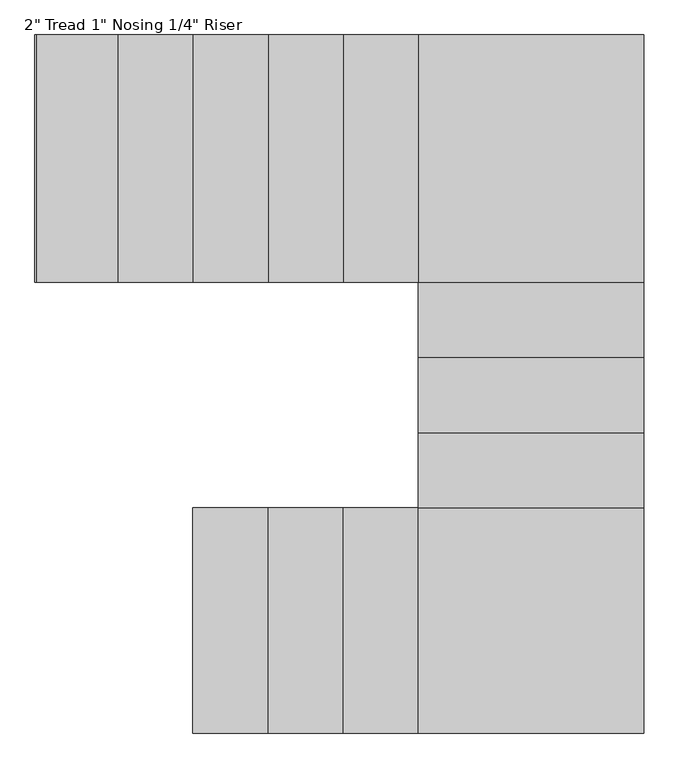
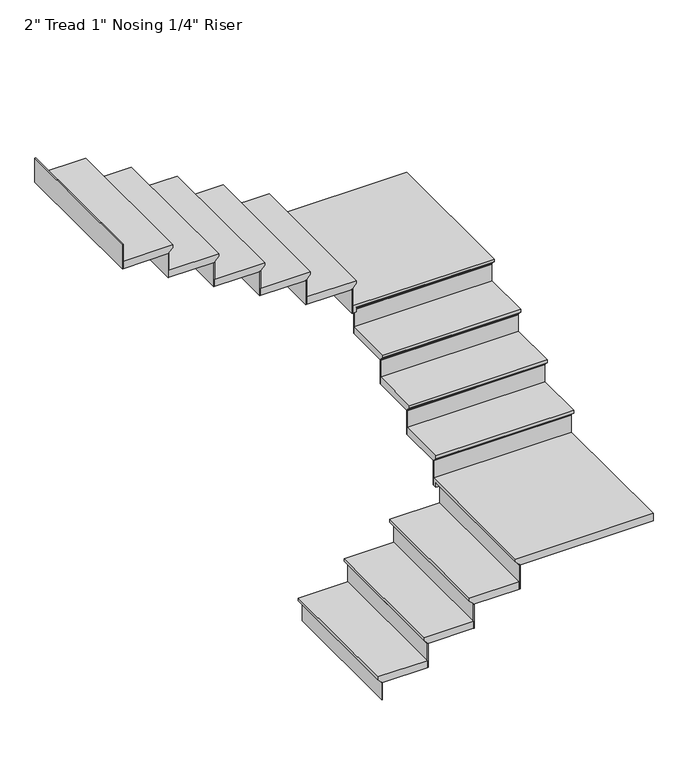
"""IFC4 building model written with IfcOpenShell, lengths in millimetres: stair flight geometry."""

from ifc_helpers import new_model, si_unit, origin, place, context, project, spatial, faceted_brep, source, transform, mapped, element, save


def stair_flight_4ba9adf8(model_context):
    return source(origin(), model_context, "Body", "Brep", [
        faceted_brep([(938.5174794, -182.0870507, 9751.4833333), (938.5174794, -182.0870507, 9770.5333333), (938.5174794, 732.3129493, 9770.5333333), (938.5174794, 732.3129493, 9751.4833333), (963.9174794, -182.0870507, 9726.0833333), (963.9174794, 732.3129493, 9726.0833333), (1268.7174794, -182.0870507, 9770.5333333), (1268.7174794, 732.3129493, 9770.5333333), (963.9174794, 732.3129493, 9719.7333333), (1268.7174794, 732.3129493, 9719.7333333), (1268.7174794, -182.0870507, 9719.7333333), (963.9174794, -182.0870507, 9719.7333333)], [[[0, 1, 2, 3]], [[4, 0, 3, 5]], [[2, 1, 6, 7]], [[8, 9, 10, 11]], [[2, 7, 9, 8, 5, 3]], [[8, 11, 4, 5]], [[6, 1, 0, 4, 11, 10]], [[7, 6, 10, 9]]]),
        faceted_brep([(963.9174794, -182.0870507, 9719.7333333), (963.9174794, -182.0870507, 9601.2), (970.2674794, -182.0870507, 9601.2), (970.2674794, -182.0870507, 9719.7333333), (963.9174794, 732.3129493, 9719.7333333), (970.2674794, 732.3129493, 9719.7333333), (970.2674794, 732.3129493, 9601.2), (963.9174794, 732.3129493, 9601.2)], [[[0, 1, 2, 3]], [[4, 5, 6, 7]], [[1, 0, 4, 7]], [[2, 1, 7, 6]], [[3, 2, 6, 5]], [[0, 3, 5, 4]]]),
        faceted_brep([(1268.7174794, -182.0870507, 9889.0666667), (1268.7174794, -182.0870507, 9719.7333333), (1275.0674794, -182.0870507, 9719.7333333), (1275.0674794, -182.0870507, 9889.0666667), (1268.7174794, 732.3129493, 9889.0666667), (1275.0674794, 732.3129493, 9889.0666667), (1275.0674794, 732.3129493, 9719.7333333), (1268.7174794, 732.3129493, 9719.7333333)], [[[0, 1, 2, 3]], [[4, 5, 6, 7]], [[1, 0, 4, 7]], [[2, 1, 7, 6]], [[3, 2, 6, 5]], [[0, 3, 5, 4]]]),
        faceted_brep([(1243.3174794, 732.3129493, 9939.8666667), (1243.3174794, -182.0870507, 9939.8666667), (1573.5174794, -182.0870507, 9939.8666667), (1573.5174794, 732.3129493, 9939.8666667), (1268.7174794, 732.3129493, 9889.0666667), (1573.5174794, 732.3129493, 9889.0666667), (1573.5174794, -182.0870507, 9889.0666667), (1268.7174794, -182.0870507, 9889.0666667), (1268.7174794, 732.3129493, 9895.4166667), (1243.3174794, 732.3129493, 9920.8166667), (1268.7174794, -182.0870507, 9895.4166667), (1243.3174794, -182.0870507, 9920.8166667)], [[[0, 1, 2, 3]], [[4, 5, 6, 7]], [[0, 3, 5, 4, 8, 9]], [[4, 7, 10, 8]], [[2, 1, 11, 10, 7, 6]], [[3, 2, 6, 5]], [[11, 1, 0, 9]], [[10, 11, 9, 8]]]),
        faceted_brep([(1573.5174794, -182.0870507, 10058.4), (1573.5174794, -182.0870507, 9889.0666667), (1579.8674794, -182.0870507, 9889.0666667), (1579.8674794, -182.0870507, 10058.4), (1573.5174794, 732.3129493, 10058.4), (1579.8674794, 732.3129493, 10058.4), (1579.8674794, 732.3129493, 9889.0666667), (1573.5174794, 732.3129493, 9889.0666667)], [[[0, 1, 2, 3]], [[4, 5, 6, 7]], [[1, 0, 4, 7]], [[2, 1, 7, 6]], [[3, 2, 6, 5]], [[0, 3, 5, 4]]]),
        faceted_brep([(1548.1174794, 732.3129493, 10109.2), (1548.1174794, -182.0870507, 10109.2), (1878.3174794, -182.0870507, 10109.2), (1878.3174794, 732.3129493, 10109.2), (1573.5174794, 732.3129493, 10058.4), (1878.3174794, 732.3129493, 10058.4), (1878.3174794, -182.0870507, 10058.4), (1573.5174794, -182.0870507, 10058.4), (1573.5174794, 732.3129493, 10064.75), (1548.1174794, 732.3129493, 10090.15), (1573.5174794, -182.0870507, 10064.75), (1548.1174794, -182.0870507, 10090.15)], [[[0, 1, 2, 3]], [[4, 5, 6, 7]], [[0, 3, 5, 4, 8, 9]], [[4, 7, 10, 8]], [[2, 1, 11, 10, 7, 6]], [[3, 2, 6, 5]], [[11, 1, 0, 9]], [[10, 11, 9, 8]]]),
        faceted_brep([(1878.3174794, -182.0870507, 10227.7333333), (1878.3174794, -182.0870507, 10058.4), (1884.6674794, -182.0870507, 10058.4), (1884.6674794, -182.0870507, 10227.7333333), (1878.3174794, 732.3129493, 10227.7333333), (1884.6674794, 732.3129493, 10227.7333333), (1884.6674794, 732.3129493, 10058.4), (1878.3174794, 732.3129493, 10058.4)], [[[0, 1, 2, 3]], [[4, 5, 6, 7]], [[1, 0, 4, 7]], [[2, 1, 7, 6]], [[3, 2, 6, 5]], [[0, 3, 5, 4]]]),
        faceted_brep([(2767.3174794, -182.0870507, 10278.5333333), (2767.3174794, 757.7129493, 10278.5333333), (1852.9174794, 757.7129493, 10278.5333333), (1852.9174794, -182.0870507, 10278.5333333), (1852.9174794, 732.3129493, 10227.7333333), (1852.9174794, 757.7129493, 10227.7333333), (2767.3174794, 757.7129493, 10227.7333333), (2767.3174794, -182.0870507, 10227.7333333), (1878.3174794, -182.0870507, 10227.7333333), (1878.3174794, 732.3129493, 10227.7333333), (1852.9174794, 732.3129493, 10259.4833333), (1852.9174794, -182.0870507, 10259.4833333), (1878.3174794, 732.3129493, 10234.0833333), (1878.3174794, -182.0870507, 10234.0833333)], [[[0, 1, 2, 3]], [[4, 5, 6, 7, 8, 9]], [[3, 2, 5, 4, 10, 11]], [[4, 9, 12, 10]], [[9, 8, 13, 12]], [[0, 3, 11, 13, 8, 7]], [[1, 0, 7, 6]], [[2, 1, 6, 5]], [[13, 11, 10, 12]]]),
        faceted_brep([(2767.3174794, 757.7129493, 10397.0666667), (2767.3174794, 757.7129493, 10227.7333333), (2767.3174794, 764.0629493, 10227.7333333), (2767.3174794, 764.0629493, 10397.0666667), (1852.9174794, 757.7129493, 10397.0666667), (1852.9174794, 764.0629493, 10397.0666667), (1852.9174794, 764.0629493, 10227.7333333), (1852.9174794, 757.7129493, 10227.7333333)], [[[0, 1, 2, 3]], [[4, 5, 6, 7]], [[1, 0, 4, 7]], [[2, 1, 7, 6]], [[3, 2, 6, 5]], [[0, 3, 5, 4]]]),
        faceted_brep([(1852.9174794, 732.3129493, 10447.8666667), (2767.3174794, 732.3129493, 10447.8666667), (2767.3174794, 1062.5129493, 10447.8666667), (1852.9174794, 1062.5129493, 10447.8666667), (1852.9174794, 757.7129493, 10397.0666667), (1852.9174794, 1062.5129493, 10397.0666667), (2767.3174794, 1062.5129493, 10397.0666667), (2767.3174794, 757.7129493, 10397.0666667), (1852.9174794, 757.7129493, 10403.4166667), (1852.9174794, 732.3129493, 10428.8166667), (2767.3174794, 757.7129493, 10403.4166667), (2767.3174794, 732.3129493, 10428.8166667)], [[[0, 1, 2, 3]], [[4, 5, 6, 7]], [[0, 3, 5, 4, 8, 9]], [[4, 7, 10, 8]], [[2, 1, 11, 10, 7, 6]], [[3, 2, 6, 5]], [[11, 1, 0, 9]], [[10, 11, 9, 8]]]),
        faceted_brep([(2767.3174794, 1062.5129493, 10566.4), (2767.3174794, 1062.5129493, 10397.0666667), (2767.3174794, 1068.8629493, 10397.0666667), (2767.3174794, 1068.8629493, 10566.4), (1852.9174794, 1062.5129493, 10566.4), (1852.9174794, 1068.8629493, 10566.4), (1852.9174794, 1068.8629493, 10397.0666667), (1852.9174794, 1062.5129493, 10397.0666667)], [[[0, 1, 2, 3]], [[4, 5, 6, 7]], [[1, 0, 4, 7]], [[2, 1, 7, 6]], [[3, 2, 6, 5]], [[0, 3, 5, 4]]]),
        faceted_brep([(1852.9174794, 1037.1129493, 10617.2), (2767.3174794, 1037.1129493, 10617.2), (2767.3174794, 1367.3129493, 10617.2), (1852.9174794, 1367.3129493, 10617.2), (1852.9174794, 1062.5129493, 10566.4), (1852.9174794, 1367.3129493, 10566.4), (2767.3174794, 1367.3129493, 10566.4), (2767.3174794, 1062.5129493, 10566.4), (1852.9174794, 1062.5129493, 10572.75), (1852.9174794, 1037.1129493, 10598.15), (2767.3174794, 1062.5129493, 10572.75), (2767.3174794, 1037.1129493, 10598.15)], [[[0, 1, 2, 3]], [[4, 5, 6, 7]], [[0, 3, 5, 4, 8, 9]], [[4, 7, 10, 8]], [[2, 1, 11, 10, 7, 6]], [[3, 2, 6, 5]], [[11, 1, 0, 9]], [[10, 11, 9, 8]]]),
        faceted_brep([(2767.3174794, 1367.3129493, 10735.7333333), (2767.3174794, 1367.3129493, 10566.4), (2767.3174794, 1373.6629493, 10566.4), (2767.3174794, 1373.6629493, 10735.7333333), (1852.9174794, 1367.3129493, 10735.7333333), (1852.9174794, 1373.6629493, 10735.7333333), (1852.9174794, 1373.6629493, 10566.4), (1852.9174794, 1367.3129493, 10566.4)], [[[0, 1, 2, 3]], [[4, 5, 6, 7]], [[1, 0, 4, 7]], [[2, 1, 7, 6]], [[3, 2, 6, 5]], [[0, 3, 5, 4]]]),
        faceted_brep([(1852.9174794, 1341.9129493, 10786.5333333), (2767.3174794, 1341.9129493, 10786.5333333), (2767.3174794, 1672.1129493, 10786.5333333), (1852.9174794, 1672.1129493, 10786.5333333), (1852.9174794, 1367.3129493, 10735.7333333), (1852.9174794, 1672.1129493, 10735.7333333), (2767.3174794, 1672.1129493, 10735.7333333), (2767.3174794, 1367.3129493, 10735.7333333), (1852.9174794, 1367.3129493, 10742.0833333), (1852.9174794, 1341.9129493, 10767.4833333), (2767.3174794, 1367.3129493, 10742.0833333), (2767.3174794, 1341.9129493, 10767.4833333)], [[[0, 1, 2, 3]], [[4, 5, 6, 7]], [[0, 3, 5, 4, 8, 9]], [[4, 7, 10, 8]], [[2, 1, 11, 10, 7, 6]], [[3, 2, 6, 5]], [[11, 1, 0, 9]], [[10, 11, 9, 8]]]),
        faceted_brep([(2767.3174794, 1672.1129493, 10905.0666667), (2767.3174794, 1672.1129493, 10735.7333333), (2767.3174794, 1678.4629493, 10735.7333333), (2767.3174794, 1678.4629493, 10905.0666667), (1852.9174794, 1672.1129493, 10905.0666667), (1852.9174794, 1678.4629493, 10905.0666667), (1852.9174794, 1678.4629493, 10735.7333333), (1852.9174794, 1672.1129493, 10735.7333333)], [[[0, 1, 2, 3]], [[4, 5, 6, 7]], [[1, 0, 4, 7]], [[2, 1, 7, 6]], [[3, 2, 6, 5]], [[0, 3, 5, 4]]]),
        faceted_brep([(2767.3174794, 2650.0129493, 10955.8666667), (1827.5174794, 2650.0129493, 10955.8666667), (1827.5174794, 1646.7129493, 10955.8666667), (2767.3174794, 1646.7129493, 10955.8666667), (1852.9174794, 1646.7129493, 10905.0666667), (1827.5174794, 1646.7129493, 10905.0666667), (1827.5174794, 2650.0129493, 10905.0666667), (2767.3174794, 2650.0129493, 10905.0666667), (2767.3174794, 1672.1129493, 10905.0666667), (1852.9174794, 1672.1129493, 10905.0666667), (1852.9174794, 1646.7129493, 10936.8166667), (2767.3174794, 1646.7129493, 10936.8166667), (1852.9174794, 1672.1129493, 10911.4166667), (2767.3174794, 1672.1129493, 10911.4166667)], [[[0, 1, 2, 3]], [[4, 5, 6, 7, 8, 9]], [[3, 2, 5, 4, 10, 11]], [[4, 9, 12, 10]], [[9, 8, 13, 12]], [[0, 3, 11, 13, 8, 7]], [[1, 0, 7, 6]], [[2, 1, 6, 5]], [[13, 11, 10, 12]]]),
        faceted_brep([(1827.5174794, 2650.0129493, 11074.4), (1827.5174794, 2650.0129493, 10905.0666667), (1821.1674794, 2650.0129493, 10905.0666667), (1821.1674794, 2650.0129493, 11074.4), (1827.5174794, 1646.7129493, 11074.4), (1821.1674794, 1646.7129493, 11074.4), (1821.1674794, 1646.7129493, 10905.0666667), (1827.5174794, 1646.7129493, 10905.0666667)], [[[0, 1, 2, 3]], [[4, 5, 6, 7]], [[1, 0, 4, 7]], [[2, 1, 7, 6]], [[3, 2, 6, 5]], [[0, 3, 5, 4]]]),
        faceted_brep([(1852.9174794, 1646.7129493, 11125.2), (1852.9174794, 2650.0129493, 11125.2), (1522.7174794, 2650.0129493, 11125.2), (1522.7174794, 1646.7129493, 11125.2), (1827.5174794, 1646.7129493, 11074.4), (1522.7174794, 1646.7129493, 11074.4), (1522.7174794, 2650.0129493, 11074.4), (1827.5174794, 2650.0129493, 11074.4), (1827.5174794, 1646.7129493, 11080.75), (1852.9174794, 1646.7129493, 11106.15), (1827.5174794, 2650.0129493, 11080.75), (1852.9174794, 2650.0129493, 11106.15)], [[[0, 1, 2, 3]], [[4, 5, 6, 7]], [[0, 3, 5, 4, 8, 9]], [[4, 7, 10, 8]], [[2, 1, 11, 10, 7, 6]], [[3, 2, 6, 5]], [[11, 1, 0, 9]], [[10, 11, 9, 8]]]),
        faceted_brep([(1522.7174794, 2650.0129493, 11243.7333333), (1522.7174794, 2650.0129493, 11074.4), (1516.3674794, 2650.0129493, 11074.4), (1516.3674794, 2650.0129493, 11243.7333333), (1522.7174794, 1646.7129493, 11243.7333333), (1516.3674794, 1646.7129493, 11243.7333333), (1516.3674794, 1646.7129493, 11074.4), (1522.7174794, 1646.7129493, 11074.4)], [[[0, 1, 2, 3]], [[4, 5, 6, 7]], [[1, 0, 4, 7]], [[2, 1, 7, 6]], [[3, 2, 6, 5]], [[0, 3, 5, 4]]]),
        faceted_brep([(1548.1174794, 1646.7129493, 11294.5333333), (1548.1174794, 2650.0129493, 11294.5333333), (1217.9174794, 2650.0129493, 11294.5333333), (1217.9174794, 1646.7129493, 11294.5333333), (1522.7174794, 1646.7129493, 11243.7333333), (1217.9174794, 1646.7129493, 11243.7333333), (1217.9174794, 2650.0129493, 11243.7333333), (1522.7174794, 2650.0129493, 11243.7333333), (1522.7174794, 1646.7129493, 11250.0833333), (1548.1174794, 1646.7129493, 11275.4833333), (1522.7174794, 2650.0129493, 11250.0833333), (1548.1174794, 2650.0129493, 11275.4833333)], [[[0, 1, 2, 3]], [[4, 5, 6, 7]], [[0, 3, 5, 4, 8, 9]], [[4, 7, 10, 8]], [[2, 1, 11, 10, 7, 6]], [[3, 2, 6, 5]], [[11, 1, 0, 9]], [[10, 11, 9, 8]]]),
        faceted_brep([(1217.9174794, 2650.0129493, 11413.0666667), (1217.9174794, 2650.0129493, 11243.7333333), (1211.5674794, 2650.0129493, 11243.7333333), (1211.5674794, 2650.0129493, 11413.0666667), (1217.9174794, 1646.7129493, 11413.0666667), (1211.5674794, 1646.7129493, 11413.0666667), (1211.5674794, 1646.7129493, 11243.7333333), (1217.9174794, 1646.7129493, 11243.7333333)], [[[0, 1, 2, 3]], [[4, 5, 6, 7]], [[1, 0, 4, 7]], [[2, 1, 7, 6]], [[3, 2, 6, 5]], [[0, 3, 5, 4]]]),
        faceted_brep([(1243.3174794, 1646.7129493, 11463.8666667), (1243.3174794, 2650.0129493, 11463.8666667), (913.1174794, 2650.0129493, 11463.8666667), (913.1174794, 1646.7129493, 11463.8666667), (1217.9174794, 1646.7129493, 11413.0666667), (913.1174794, 1646.7129493, 11413.0666667), (913.1174794, 2650.0129493, 11413.0666667), (1217.9174794, 2650.0129493, 11413.0666667), (1217.9174794, 1646.7129493, 11419.4166667), (1243.3174794, 1646.7129493, 11444.8166667), (1217.9174794, 2650.0129493, 11419.4166667), (1243.3174794, 2650.0129493, 11444.8166667)], [[[0, 1, 2, 3]], [[4, 5, 6, 7]], [[0, 3, 5, 4, 8, 9]], [[4, 7, 10, 8]], [[2, 1, 11, 10, 7, 6]], [[3, 2, 6, 5]], [[11, 1, 0, 9]], [[10, 11, 9, 8]]]),
        faceted_brep([(913.1174794, 2650.0129493, 11582.4), (913.1174794, 2650.0129493, 11413.0666667), (906.7674794, 2650.0129493, 11413.0666667), (906.7674794, 2650.0129493, 11582.4), (913.1174794, 1646.7129493, 11582.4), (906.7674794, 1646.7129493, 11582.4), (906.7674794, 1646.7129493, 11413.0666667), (913.1174794, 1646.7129493, 11413.0666667)], [[[0, 1, 2, 3]], [[4, 5, 6, 7]], [[1, 0, 4, 7]], [[2, 1, 7, 6]], [[3, 2, 6, 5]], [[0, 3, 5, 4]]]),
        faceted_brep([(938.5174794, 1646.7129493, 11633.2), (938.5174794, 2650.0129493, 11633.2), (608.3174794, 2650.0129493, 11633.2), (608.3174794, 1646.7129493, 11633.2), (913.1174794, 1646.7129493, 11582.4), (608.3174794, 1646.7129493, 11582.4), (608.3174794, 2650.0129493, 11582.4), (913.1174794, 2650.0129493, 11582.4), (913.1174794, 1646.7129493, 11588.75), (938.5174794, 1646.7129493, 11614.15), (913.1174794, 2650.0129493, 11588.75), (938.5174794, 2650.0129493, 11614.15)], [[[0, 1, 2, 3]], [[4, 5, 6, 7]], [[0, 3, 5, 4, 8, 9]], [[4, 7, 10, 8]], [[2, 1, 11, 10, 7, 6]], [[3, 2, 6, 5]], [[11, 1, 0, 9]], [[10, 11, 9, 8]]]),
        faceted_brep([(608.3174794, 2650.0129493, 11751.7333333), (608.3174794, 2650.0129493, 11582.4), (601.9674794, 2650.0129493, 11582.4), (601.9674794, 2650.0129493, 11751.7333333), (608.3174794, 1646.7129493, 11751.7333333), (601.9674794, 1646.7129493, 11751.7333333), (601.9674794, 1646.7129493, 11582.4), (608.3174794, 1646.7129493, 11582.4)], [[[0, 1, 2, 3]], [[4, 5, 6, 7]], [[1, 0, 4, 7]], [[2, 1, 7, 6]], [[3, 2, 6, 5]], [[0, 3, 5, 4]]]),
        faceted_brep([(303.5174794, 2650.0129493, 11921.0666667), (303.5174794, 2650.0129493, 11751.7333333), (297.1674794, 2650.0129493, 11751.7333333), (297.1674794, 2650.0129493, 11921.0666667), (303.5174794, 1646.7129493, 11921.0666667), (297.1674794, 1646.7129493, 11921.0666667), (297.1674794, 1646.7129493, 11751.7333333), (303.5174794, 1646.7129493, 11751.7333333)], [[[0, 1, 2, 3]], [[4, 5, 6, 7]], [[1, 0, 4, 7]], [[2, 1, 7, 6]], [[3, 2, 6, 5]], [[0, 3, 5, 4]]]),
        faceted_brep([(633.7174794, 1646.7129493, 11802.5333333), (633.7174794, 2650.0129493, 11802.5333333), (303.5174794, 2650.0129493, 11802.5333333), (303.5174794, 1646.7129493, 11802.5333333), (608.3174794, 1646.7129493, 11751.7333333), (303.5174794, 1646.7129493, 11751.7333333), (303.5174794, 2650.0129493, 11751.7333333), (608.3174794, 2650.0129493, 11751.7333333), (608.3174794, 1646.7129493, 11758.0833333), (633.7174794, 1646.7129493, 11783.4833333), (608.3174794, 2650.0129493, 11758.0833333), (633.7174794, 2650.0129493, 11783.4833333)], [[[0, 1, 2, 3]], [[4, 5, 6, 7]], [[0, 3, 5, 4, 8, 9]], [[4, 7, 10, 8]], [[2, 1, 11, 10, 7, 6]], [[3, 2, 6, 5]], [[11, 1, 0, 9]], [[10, 11, 9, 8]]]),
    ])


if __name__ == "__main__":
    model = new_model("IFC4")
    model_context = context("Model", 3, world=origin())
    ifc_project = project(units=[si_unit("LENGTHUNIT", "METRE", prefix="MILLI")], contexts=[model_context])
    site = spatial("IfcSite", under=ifc_project)
    building = spatial("IfcBuilding", under=site)
    placement = place(None, origin())
    stair_flight_shape = stair_flight_4ba9adf8(model_context)
    element("IfcStairFlight", 1, ObjectType="2\" Tread 1\" Nosing 1/4\" Riser", at=placement, inside=building, context=model_context, shape_type="MappedRepresentation", body=[
        mapped(stair_flight_shape, transform((0.0, 0.0, 0.0), x_axis=(1.0, 0.0, 0.0), y_axis=(0.0, 1.0, 0.0), z_axis=(0.0, 0.0, 1.0))),
    ])
    save(model, "model.ifc")
